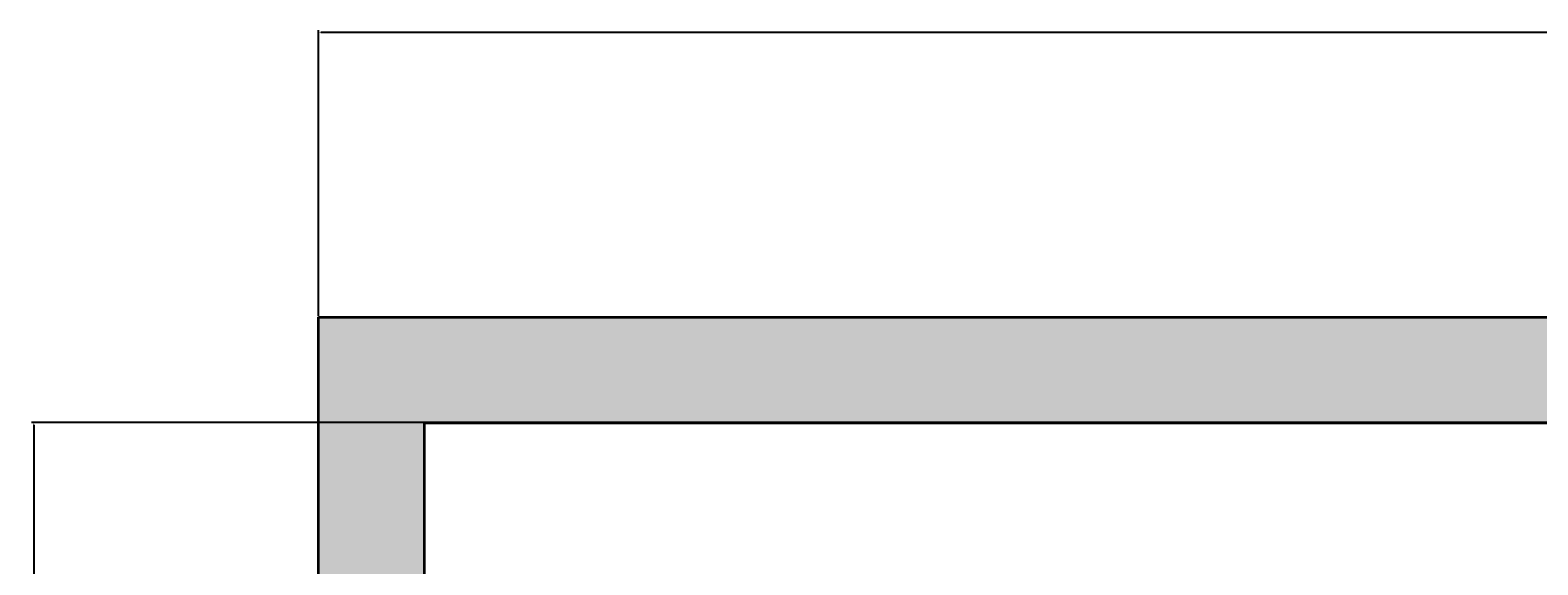
# Model space of a CAD drawing. Units: millimetres. Extents: x 2817 to 5038, y 1110 to 3565.
# Tile 17 of 21: x 2817 to 2946, y 1593 to 1639. Entities that reach past the tile are written whole.
import ezdxf

# ---------------------------------------------------------------- set-up
doc = ezdxf.new("R2010")
doc.units = ezdxf.units.MM
doc.layers.add('A-ANNO-DIMS', color=2, linetype='Continuous', lineweight=18)
doc.layers.add('A-WALL', color=7, linetype='Continuous', lineweight=35)
doc.layers.add('A-WALL-PATT', color=51, linetype='Continuous', lineweight=13, true_color=0xf7f281)
doc.styles.get("Standard").update_dxf_attribs({"font": 'arial.ttf'})
doc.dimstyles.get("Standard").update_dxf_attribs({"dimtxt": 0.18, "dimasz": 0.18, "dimexe": 0.18, "dimexo": 0.0625, "dimgap": 0.09, "dimtad": 0, "dimtih": 1, "dimtoh": 1, "dimdec": 4, "dimzin": 0, "dimdsep": 46, "dimtxsty": 'Standard', "dimcen": 0.09, "dimadec": 0, "dimazin": 0, "dimtfac": 1, "dimtdec": 4, "dimtofl": 0, "dimtmove": 0, "dimatfit": 3, "dimfxl": 1, "dimtolj": 1, "dimtzin": 0, "dimarcsym": 0})

# ---------------------------------------------------------------- blocks, each defined once
blk = doc.blocks.new('*D26')
at = {"layer": 'A-ANNO-DIMS', "color": 0, "lineweight": -2, "transparency": 16777216}
for p, q in [((2841.74, 1614.5), (2841.74, 1638.87)), ((2841.92, 1638.69), (3013.95, 1638.69)), ((3186.56, 1638.69), (3014.53, 1638.69)), ((3186.74, 1614.5), (3186.74, 1638.87))]:
    blk.add_line(p, q, dxfattribs=at)
for points in [[(2841.92, 1638.72), (2841.92, 1638.66), (2841.74, 1638.69)], [(3186.56, 1638.72), (3186.56, 1638.66), (3186.74, 1638.69)]]:
    blk.add_solid(points, dxfattribs=at)
at = {"layer": 'Defpoints', "color": 0, "lineweight": -2, "transparency": 16777216}
for p in [(3186.74, 1638.69), (2841.74, 1614.44), (3186.74, 1614.44)]:
    blk.add_point(p, dxfattribs=at)
at = {"layer": 'A-ANNO-DIMS', "color": 0, "transparency": 16777216, "insert": (3014.24, 1638.69), "char_height": 0.18, "attachment_point": 5}
blk.add_mtext('\\A1;345', dxfattribs=at)
blk = doc.blocks.new('*D39')
at = {"layer": 'A-ANNO-DIMS', "color": 0, "lineweight": -2, "transparency": 16777216}
for p, q in [((3105.68, 1605.44), (2817.31, 1605.44)), ((2817.49, 1605.26), (2817.49, 1589.62)), ((2817.49, 1573.62), (2817.49, 1589.25)), ((3110.18, 1573.44), (2817.31, 1573.44))]:
    blk.add_line(p, q, dxfattribs=at)
for points in [[(2817.46, 1605.26), (2817.52, 1605.26), (2817.49, 1605.44)], [(2817.46, 1573.62), (2817.52, 1573.62), (2817.49, 1573.44)]]:
    blk.add_solid(points, dxfattribs=at)
at = {"layer": 'Defpoints', "color": 0, "lineweight": -2, "transparency": 16777216}
for p in [(2817.49, 1605.44), (3105.74, 1605.44), (3110.24, 1573.44)]:
    blk.add_point(p, dxfattribs=at)
at = {"layer": 'A-ANNO-DIMS', "color": 0, "transparency": 16777216, "insert": (2817.49, 1589.44), "char_height": 0.18, "attachment_point": 5}
blk.add_mtext('\\A1;32', dxfattribs=at)
blk = doc.blocks.new('*D46')
at = {"layer": 'A-ANNO-DIMS', "color": 0, "lineweight": -2, "transparency": 16777216}
for p, q in [((3052.18, 1605.44), (2817.31, 1605.44)), ((2817.49, 1605.26), (2817.49, 1589.79)), ((2817.49, 1573.96), (2817.49, 1589.43)), ((3052.08, 1573.78), (2817.31, 1573.78))]:
    blk.add_line(p, q, dxfattribs=at)
for points in [[(2817.46, 1605.26), (2817.52, 1605.26), (2817.49, 1605.44)], [(2817.46, 1573.96), (2817.52, 1573.96), (2817.49, 1573.78)]]:
    blk.add_solid(points, dxfattribs=at)
at = {"layer": 'Defpoints', "color": 0, "lineweight": -2, "transparency": 16777216}
for p in [(2817.49, 1605.44), (3052.24, 1605.44), (3052.14, 1573.78)]:
    blk.add_point(p, dxfattribs=at)
at = {"layer": 'A-ANNO-DIMS', "color": 0, "transparency": 16777216, "insert": (2817.49, 1589.61), "char_height": 0.18, "attachment_point": 5}
blk.add_mtext('\\A1;31.65', dxfattribs=at)

msp = doc.modelspace()

# ---------------------------------------------------------------- hatches: boundary and pattern name
at = {"layer": 'A-WALL-PATT'}
h = msp.add_hatch(color=256, dxfattribs=at)
h.dxf.hatch_style = 1
h.paths.add_polyline_path([(3186.7393, 1614.4357), (2841.7393, 1614.4357), (2841.7393, 1568.614), (2850.7393, 1568.7609), (2850.7393, 1605.4357), (2982.7393, 1605.4357), (2991.7393, 1605.4357), (3052.2393, 1605.4357), (3052.2393, 1573.7835), (3061.2393, 1573.7835), (3061.2393, 1605.4357), (3182.2393, 1605.4357), (3182.2393, 1143.4357), (3181.2393, 1143.4357), (3181.2393, 1134.4357), (3186.7393, 1134.4357)])
h.paths.add_polyline_path([(3061.2393, 1143.4357), (3061.2393, 1147.4357), (3052.2393, 1147.4357), (3052.2393, 1143.4357), (2850.7393, 1143.4357), (2850.7393, 1145.2996), (2841.7393, 1145.2996), (2841.7393, 1134.4357), (3061.2393, 1134.4357)], flags=17)
h.paths.add_polyline_path([(2850.7393, 1265.4357), (2946.7393, 1265.4357), (2946.7393, 1270.8357), (2946.7393, 1274.4357), (2850.7393, 1274.4357), (2850.7381, 1274.4357), (2850.7381, 1274.2564), (2841.7393, 1274.2564), (2841.7393, 1193.1527), (2850.7393, 1193.2996)], flags=17)
h.paths.add_polyline_path([(3061.2393, 1299.098), (3052.2393, 1299.098), (3052.2393, 1274.4357), (2991.7393, 1274.4357), (2991.7393, 1340.4357), (2982.7393, 1340.4357), (2982.7393, 1274.4357), (2982.7393, 1265.4357), (3052.2393, 1265.4357), (3052.2393, 1259.143), (3061.2393, 1259.2899)], flags=17)
h.paths.add_polyline_path([(3061.2393, 1383.4357), (3052.2393, 1383.4357), (3052.2393, 1379.4357), (2931.7393, 1379.4357), (2922.7393, 1379.4357), (2850.7393, 1379.4357), (2850.7381, 1379.4357), (2850.7381, 1379.3646), (2841.7393, 1379.3646), (2841.7393, 1322.1095), (2850.7393, 1322.2564), (2850.7393, 1370.4357), (2982.7393, 1370.4357), (2987.2393, 1370.4357), (3017.2393, 1370.4357), (3052.2393, 1370.4357), (3052.2393, 1323.098), (3061.2393, 1323.098)], flags=17)

# ---------------------------------------------------------------- linework, layer by layer
at = {"layer": 'A-WALL'}
for p, q in [((2841.7393, 1614.4357), (3186.7393, 1614.4357)), ((2841.7393, 1134.4357), (2841.7393, 1614.4357)), ((2850.7393, 1605.4357), (2982.7393, 1605.4357)), ((2850.7393, 1509.4357), (2850.7393, 1605.4357))]:
    msp.add_line(p, q, dxfattribs=at)

# ---------------------------------------------------------------- dimensions: what is measured, and where the dimension line sits
at = {"layer": 'A-ANNO-DIMS'}
dim = msp.add_linear_dim(base=(3186.7393, 1638.6857), p1=(2841.7393, 1614.4357), p2=(3186.7393, 1614.4357), dimstyle='Standard', override={"dimdec": 0, "dimlfac": 1, "dimrnd": 0, "dimzin": 0, "dimdsep": 46, "dimlunit": 2}, dxfattribs=at)
dim.commit()
dim.dimension.update_dxf_attribs({"geometry": '*D26', "text_midpoint": (3014.2393, 1638.6857)})
for p1, p2, override, picture, middle in [((3052.1378, 1573.7835), (3052.2393, 1605.4357), {"dimdec": 2, "dimlfac": 1, "dimrnd": 0, "dimzin": 0, "dimdsep": 46, "dimlunit": 2}, '*D46', (2817.4881, 1589.6096)), ((3110.2393, 1573.4357), (3105.7393, 1605.4357), {"dimdec": 0, "dimlfac": 1, "dimrnd": 0, "dimzin": 0, "dimdsep": 46, "dimlunit": 2}, '*D39', (2817.4881, 1589.4357))]:
    dim = msp.add_linear_dim(base=(2817.4881, 1605.4357), p1=p1, p2=p2, angle=90, dimstyle='Standard', override=override, dxfattribs=at)
    dim.commit()
    dim.dimension.update_dxf_attribs({"geometry": picture, "text_midpoint": middle})

doc.saveas('drawing.dxf')
